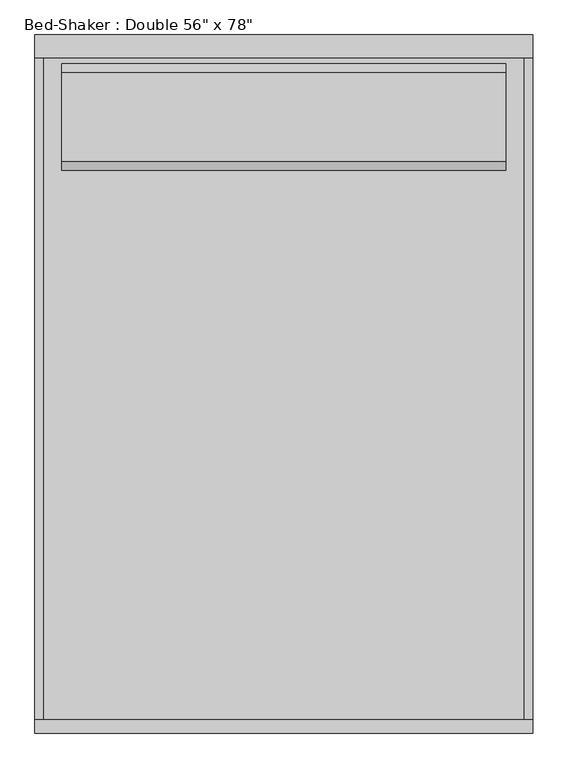
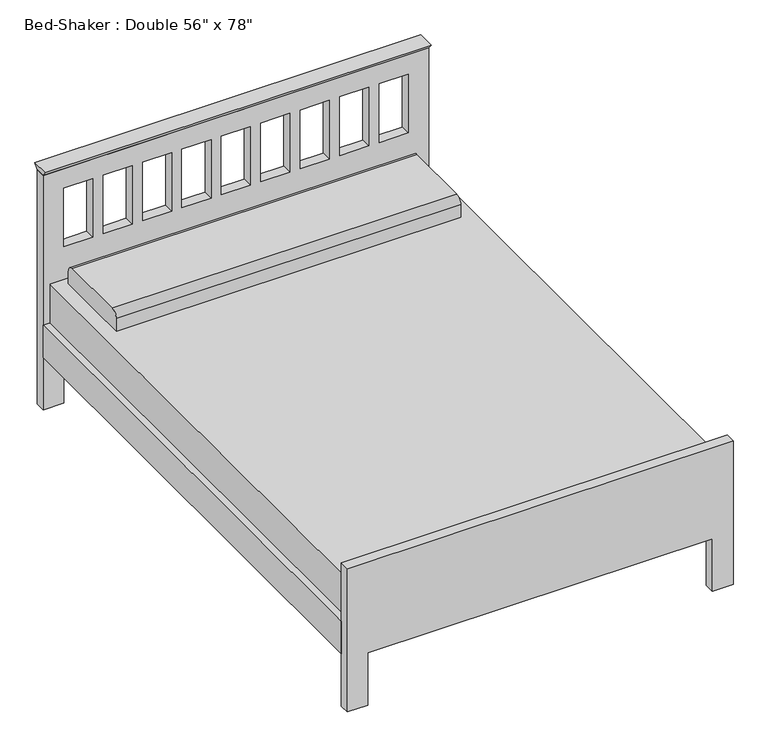
"""IFC4 building model written with IfcOpenShell, lengths in millimetres: furniture geometry."""

from ifc_helpers import new_model, si_unit, point, frame, frame_2d, origin, place, context, project, spatial, polyline, circle_curve, trimmed, segment, composite_curve, outline, extrude, source, transform, mapped, element, save


def furniture_121fd3aa(model_context):
    return source(origin(), model_context, "Body", "SweptSolid", [
        extrude(outline(polyline([(914.4, 692.4168067), (914.4, -730.0365546), (0.0, -730.0365546), (0.0, -654.05), (203.2, -654.05), (203.2, 615.95), (0.0, 615.95), (0.0, 692.4168067), (914.4, 692.4168067)]), holes=[polyline([(838.2, -546.8055556), (609.6, -546.8055556), (609.6, -654.05), (838.2, -654.05), (838.2, -546.8055556)]), polyline([(838.2, -401.4611111), (609.6, -401.4611111), (609.6, -508.7055556), (838.2, -508.7055556), (838.2, -401.4611111)]), polyline([(838.2, -256.1166667), (609.6, -256.1166667), (609.6, -363.3611111), (838.2, -363.3611111), (838.2, -256.1166667)]), polyline([(838.2, -110.7722222), (609.6, -110.7722222), (609.6, -218.0166667), (838.2, -218.0166667), (838.2, -110.7722222)]), polyline([(838.2, 179.9166667), (609.6, 179.9166667), (609.6, 72.6722222), (838.2, 72.6722222), (838.2, 179.9166667)]), polyline([(838.2, 325.2611111), (609.6, 325.2611111), (609.6, 218.0166667), (838.2, 218.0166667), (838.2, 325.2611111)]), polyline([(838.2, 470.6055556), (609.6, 470.6055556), (609.6, 363.3611111), (838.2, 363.3611111), (838.2, 470.6055556)]), polyline([(838.2, 615.95), (609.6, 615.95), (609.6, 508.7055556), (838.2, 508.7055556), (838.2, 615.95)]), polyline([(838.2, 34.5722222), (609.6, 34.5722222), (609.6, -72.6722222), (838.2, -72.6722222), (838.2, 34.5722222)])]), frame((0.0, -38.1, 0.0), z_axis=(0.0, 1.0, 0.0), x_axis=(0.0, 0.0, 1.0)), (0.0, 0.0, 1.0), 38.1),
        extrude(outline(polyline([(0.0, -654.05), (203.2, -654.05), (203.2, 615.95), (0.0, 615.95), (0.0, 692.15), (558.8, 692.15), (558.8, -730.25), (0.0, -730.25), (0.0, -654.05)])), frame((0.0, -1981.2, 0.0), z_axis=(0.0, 1.0, 0.0), x_axis=(0.0, 0.0, 1.0)), (0.0, 0.0, 1.0), 38.1),
        extrude(outline(polyline([(-730.25, -1943.1), (-730.25, -38.1), (-704.85, -38.1), (-704.85, -1943.1), (-730.25, -1943.1)])), frame((0.0, 0.0, 203.5755296), z_axis=(0.0, 0.0, 1.0), x_axis=(1.0, 0.0, 0.0)), (0.0, 0.0, 1.0), 127.0),
        extrude(outline(polyline([(666.75, -1943.1), (666.75, -38.1), (692.15, -38.1), (692.15, -1943.1), (666.75, -1943.1)])), frame((0.0, 0.0, 203.0994861), z_axis=(0.0, 0.0, 1.0), x_axis=(1.0, 0.0, 0.0)), (0.0, 0.0, 1.0), 127.0),
        extrude(outline(polyline([(666.75, -38.1), (666.75, -1943.1), (-704.85, -1943.1), (-704.85, -38.1), (666.75, -38.1)])), frame((0.0, 0.0, 228.6), z_axis=(0.0, 0.0, 1.0), x_axis=(1.0, 0.0, 0.0)), (0.0, 0.0, 1.0), 254.0),
        extrude(outline(composite_curve([segment(polyline([(-373.2486637, 482.6), (-373.2486637, 533.4)]), True, "CONTINUOUS"), segment(trimmed(circle_curve(frame_2d((-347.8486637, 533.4)), 25.4), [point((-373.2486637, 533.4))], [point((-347.8486637, 558.8))], False, "CARTESIAN"), True, "CONTINUOUS"), segment(polyline([(-347.8486637, 558.8), (-93.8486637, 558.8)]), True, "CONTINUOUS"), segment(trimmed(circle_curve(frame_2d((-93.8486637, 533.4)), 25.4), [point((-93.8486637, 558.8))], [point((-68.4486637, 533.4))], False, "CARTESIAN"), True, "CONTINUOUS"), segment(polyline([(-68.4486637, 533.4), (-68.4486637, 482.6), (-373.2486637, 482.6)]), True, "CONTINUOUS")], self_intersect=False)), frame((-654.05, 0.0, 0.0), z_axis=(1.0, 0.0, 0.0), x_axis=(0.0, 1.0, 0.0)), (0.0, 0.0, 1.0), 1270.0),
        extrude(outline(polyline([(-38.1, 914.4), (-51.9545455, 933.45), (13.8545455, 933.45), (0.0, 914.4), (-38.1, 914.4)])), frame((-730.0365546, 0.0, 0.0), z_axis=(1.0, 0.0, 0.0), x_axis=(0.0, 1.0, 0.0)), (0.0, 0.0, 1.0), 1422.4533613),
    ])


if __name__ == "__main__":
    model = new_model("IFC4")
    model_context = context("Model", 3, world=origin())
    ifc_project = project(units=[si_unit("LENGTHUNIT", "METRE", prefix="MILLI")], contexts=[model_context])
    site = spatial("IfcSite", under=ifc_project)
    building = spatial("IfcBuilding", under=site)
    placement = place(None, origin())
    furniture_shape = furniture_121fd3aa(model_context)
    element("IfcFurniture", 1, ObjectType="Bed-Shaker : Double 56\" x 78\"", at=placement, inside=building, context=model_context, shape_type="MappedRepresentation", body=[
        mapped(furniture_shape, transform((0.0, 0.0, 0.0), x_axis=(1.0, 0.0, 0.0), y_axis=(0.0, 1.0, 0.0), z_axis=(0.0, 0.0, 1.0))),
    ])
    save(model, "model.ifc")

# Revit data of these elements
# Type "Bed-Shaker : Double 56\" x 78\""
#   Assembly Code = "E2020200"
#   Length = 6' - 6"
#   Width = 4' - 8"
#   Frame Material = Birch
#   Mattress Material = Linen, White
#   Default Elevation = 0
# Element 1 (IfcFurniture, "Bed-Shaker : Double 56\" x 78\"")
#   Materials on its faces: "Birch", "Linen, White"
# Materials
#   "Birch": class "Wood", colour RGB 224 178 126, transparency 0, Description = "Betula Alleghaniensis", Cost = 0
#   "Linen, White": class "Textile", colour RGB 247 247 239, transparency 0, Description = "Linen, white", Cost = 0
